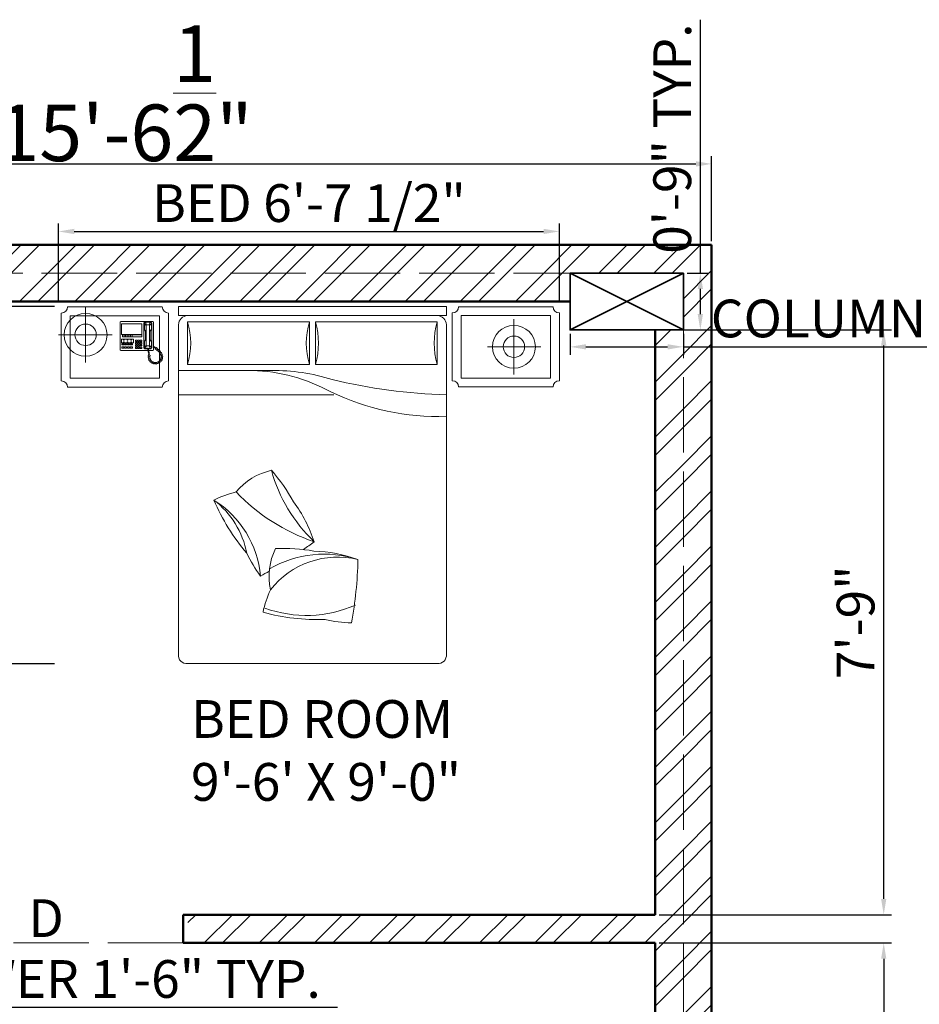
# Model space of a CAD drawing. Units: millimetres. Extents: x 4237 to 5109, y 21391 to 22486.
# Tile 12 of 17: x 4535 to 4678, y 22320 to 22477. Entities that reach past the tile are written whole.
import ezdxf

# ---------------------------------------------------------------- set-up
doc = ezdxf.new("R2010")
doc.units = ezdxf.units.MM
doc.linetypes.add('ACAD_ISO02W100', pattern=[15, 12, -3])
for name, color, linetype, lineweight in [('A-ANNO-DIMS', 2, 'Continuous', 18), ('A-ANNO-TEXT', 7, 'Continuous', 18), ('A-AREA-IDEN', 3, 'Continuous', 18), ('A-FLOR-OVHD', 1, 'ACAD_ISO02W100', 18), ('A-FURN', 8, 'Continuous', 18), ('A-WALL', 7, 'Continuous', 50), ('A-WALL-PATT', 252, 'Continuous', 13), ('column', 102, 'Continuous', 35)]:
    doc.layers.add(name, color=color, linetype=linetype, lineweight=lineweight)
doc.styles.get("Standard").update_dxf_attribs({"font": 'arial.ttf'})
doc.dimstyles.new('ISO-25', dxfattribs={"dimtxt": 6, "dimasz": 2.5, "dimexe": 1.25, "dimexo": 0.625, "dimtad": 1, "dimdec": 1, "dimlunit": 4, "dimtxsty": 'Standard', "dimcen": 2.5, "dimadec": 0, "dimazin": 0, "dimtfac": 1, "dimtdec": 1, "dimtmove": 0, "dimatfit": 3, "dimfxl": 1, "dimarcsym": 0})

# ---------------------------------------------------------------- blocks, each defined once
blk = doc.blocks.new('A$C07097A50')
for p, q in [((0.0503, 1.9981), (0.5803, 1.9981)), ((0.1513, 1.6872), (0.1513, 1.9968)), ((0.6716, 1.9489), (0.6716, 2.0001)), ((0.6716, 2.0001), (2.1719, 2.0001)), ((2.1719, 1.9489), (2.1719, 2.0001)), ((2.7701, 1.9993), (2.2401, 1.9993)), ((0.0153, 1.9631), (0.0153, 1.5831)), ((0.0653, 1.9481), (0.0653, 1.5981)), ((0.0653, 1.9481), (0.5653, 1.9481)), ((0.5653, 1.9481), (0.5653, 1.5981)), ((0.6153, 1.9631), (0.6153, 1.5831)), ((2.1719, 1.9489), (0.6716, 1.9489)), ((2.2051, 1.9643), (2.2051, 1.5843)), ((2.2551, 1.9493), (2.2551, 1.5993)), ((2.7551, 1.9493), (2.2551, 1.9493)), ((2.7551, 1.9493), (2.7551, 1.5993)), ((2.8051, 1.9643), (2.8051, 1.5843)), ((0.3481, 1.9163), (0.3458, 1.914)), ((0.3458, 1.914), (0.3458, 1.7563)), ((0.3481, 1.9163), (0.5287, 1.9163)), ((0.3526, 1.9037), (0.3526, 1.8431)), ((0.4669, 1.9037), (0.3526, 1.9037)), ((0.4669, 1.8431), (0.4669, 1.9037)), ((0.4772, 1.9071), (0.4818, 1.9129)), ((0.4772, 1.7688), (0.4772, 1.9071)), ((0.4818, 1.9094), (0.4807, 1.9049)), ((0.4807, 1.9049), (0.4807, 1.874)), ((0.4807, 1.9049), (0.4909, 1.8946)), ((0.4818, 1.9129), (0.5161, 1.9129)), ((0.4864, 1.9117), (0.4818, 1.9094)), ((0.4921, 1.8969), (0.4864, 1.9117)), ((0.4864, 1.9117), (0.5138, 1.9117)), ((0.4909, 1.8946), (0.4921, 1.8969)), ((0.4909, 1.8431), (0.4909, 1.8946)), ((0.5081, 1.8969), (0.4921, 1.8969)), ((0.5081, 1.8969), (0.5138, 1.9117)), ((0.5092, 1.8946), (0.5081, 1.8969)), ((0.5195, 1.9049), (0.5092, 1.8946)), ((0.5092, 1.8431), (0.5092, 1.8946)), ((0.5138, 1.9117), (0.5184, 1.9094)), ((0.5161, 1.9129), (0.5218, 1.9071)), ((0.5184, 1.9094), (0.5195, 1.9049)), ((0.5195, 1.9049), (0.5195, 1.874)), ((0.5218, 1.9071), (0.5218, 1.77)), ((0.5287, 1.9163), (0.5309, 1.914)), ((0.5309, 1.914), (0.5309, 1.7563)), ((0.6716, 1.8977), (0.6716, 0.0512)), ((2.1719, 0.0512), (2.1719, 1.8977)), ((2.5505, 1.6201), (2.5505, 1.9296)), ((0, 1.8416), (0.3001, 1.8416)), ((0.3526, 1.8431), (0.4669, 1.8431)), ((0.3572, 1.8409), (0.3572, 1.8294)), ((0.4669, 1.8409), (0.3572, 1.8409)), ((0.3572, 1.8294), (0.4669, 1.8294)), ((0.3664, 1.8409), (0.3664, 1.8294)), ((0.3755, 1.8409), (0.3755, 1.8294)), ((0.3846, 1.8409), (0.3846, 1.8294)), ((0.3938, 1.8409), (0.3938, 1.8294)), ((0.4029, 1.8409), (0.4029, 1.8294)), ((0.4121, 1.8409), (0.4121, 1.8294)), ((0.4669, 1.8294), (0.4669, 1.8409)), ((0.4807, 1.874), (0.4829, 1.8683)), ((0.4829, 1.8683), (0.4864, 1.8626)), ((0.4864, 1.8626), (0.4875, 1.8546)), ((0.4864, 1.8134), (0.4875, 1.8214)), ((0.4875, 1.8546), (0.4875, 1.8431)), ((0.4875, 1.8214), (0.4875, 1.8431)), ((0.4909, 1.8431), (0.4909, 1.7814)), ((0.5092, 1.8431), (0.5092, 1.7814)), ((0.5138, 1.8626), (0.5127, 1.8546)), ((0.5127, 1.8546), (0.5127, 1.8431)), ((0.5127, 1.8214), (0.5127, 1.8431)), ((0.5138, 1.8134), (0.5127, 1.8214)), ((0.5172, 1.8683), (0.5138, 1.8626)), ((0.5195, 1.874), (0.5172, 1.8683)), ((0.4201, 1.8168), (0.3526, 1.8168)), ((0.3526, 1.8168), (0.3526, 1.7963)), ((0.3526, 1.7963), (0.4201, 1.7963)), ((0.3652, 1.7906), (0.3538, 1.7906)), ((0.3538, 1.7906), (0.3538, 1.786)), ((0.3538, 1.786), (0.3652, 1.786)), ((0.3538, 1.7666), (0.3538, 1.7734)), ((0.3538, 1.7734), (0.3652, 1.7734)), ((0.3652, 1.7666), (0.3538, 1.7666)), ((0.3675, 1.8146), (0.3641, 1.8146)), ((0.3641, 1.8146), (0.3641, 1.8111)), ((0.3641, 1.8111), (0.3675, 1.8111)), ((0.3641, 1.802), (0.3641, 1.7986)), ((0.3675, 1.802), (0.3641, 1.802)), ((0.3641, 1.7986), (0.3675, 1.7986)), ((0.3652, 1.786), (0.3652, 1.7906)), ((0.3652, 1.7734), (0.3652, 1.7666)), ((0.3675, 1.8111), (0.3675, 1.8146)), ((0.3675, 1.7986), (0.3675, 1.802)), ((0.3812, 1.7906), (0.3698, 1.7906)), ((0.3698, 1.7906), (0.3698, 1.786)), ((0.3698, 1.786), (0.3812, 1.786)), ((0.3698, 1.7666), (0.3698, 1.7734)), ((0.3698, 1.7734), (0.3812, 1.7734)), ((0.3812, 1.7666), (0.3698, 1.7666)), ((0.3812, 1.786), (0.3812, 1.7906)), ((0.3812, 1.7734), (0.3812, 1.7666)), ((0.3846, 1.8146), (0.3846, 1.8111)), ((0.3881, 1.8146), (0.3846, 1.8146)), ((0.3846, 1.8111), (0.3881, 1.8111)), ((0.3846, 1.802), (0.3846, 1.7986)), ((0.3881, 1.802), (0.3846, 1.802)), ((0.3846, 1.7986), (0.3881, 1.7986)), ((0.3972, 1.7906), (0.3858, 1.7906)), ((0.3858, 1.7906), (0.3858, 1.786)), ((0.3858, 1.786), (0.3972, 1.786)), ((0.3858, 1.7666), (0.3858, 1.7734)), ((0.3858, 1.7734), (0.3972, 1.7734)), ((0.3972, 1.7666), (0.3858, 1.7666)), ((0.3881, 1.8111), (0.3881, 1.8146)), ((0.3881, 1.7986), (0.3881, 1.802)), ((0.3972, 1.786), (0.3972, 1.7906)), ((0.3972, 1.7734), (0.3972, 1.7666)), ((0.4018, 1.7906), (0.4018, 1.786)), ((0.4132, 1.7906), (0.4018, 1.7906)), ((0.4018, 1.786), (0.4132, 1.786)), ((0.4018, 1.7734), (0.4132, 1.7734)), ((0.4018, 1.7666), (0.4018, 1.7734)), ((0.4132, 1.7666), (0.4018, 1.7666)), ((0.4052, 1.8146), (0.4052, 1.8111)), ((0.4086, 1.8146), (0.4052, 1.8146)), ((0.4052, 1.8111), (0.4086, 1.8111)), ((0.4052, 1.802), (0.4052, 1.7986)), ((0.4086, 1.802), (0.4052, 1.802)), ((0.4052, 1.7986), (0.4086, 1.7986)), ((0.4086, 1.8111), (0.4086, 1.8146)), ((0.4086, 1.7986), (0.4086, 1.802)), ((0.4132, 1.786), (0.4132, 1.7906)), ((0.4132, 1.7734), (0.4132, 1.7666)), ((0.4201, 1.7963), (0.4201, 1.8168)), ((0.4304, 1.8111), (0.4395, 1.8111)), ((0.4304, 1.8043), (0.4304, 1.8111)), ((0.4395, 1.8043), (0.4304, 1.8043)), ((0.4304, 1.7986), (0.4395, 1.7986)), ((0.4304, 1.7917), (0.4304, 1.7986)), ((0.4395, 1.7917), (0.4304, 1.7917)), ((0.4304, 1.778), (0.4304, 1.7848)), ((0.4304, 1.7848), (0.4395, 1.7848)), ((0.4395, 1.778), (0.4304, 1.778)), ((0.4304, 1.7723), (0.4395, 1.7723)), ((0.4304, 1.7654), (0.4304, 1.7723)), ((0.4395, 1.8111), (0.4395, 1.8043)), ((0.4395, 1.7986), (0.4395, 1.7917)), ((0.4395, 1.7848), (0.4395, 1.778)), ((0.4395, 1.7723), (0.4395, 1.7654)), ((0.4441, 1.8043), (0.4441, 1.8111)), ((0.4441, 1.8111), (0.4532, 1.8111)), ((0.4532, 1.8043), (0.4441, 1.8043)), ((0.4441, 1.7986), (0.4532, 1.7986)), ((0.4441, 1.7917), (0.4441, 1.7986)), ((0.4532, 1.7917), (0.4441, 1.7917)), ((0.4441, 1.778), (0.4441, 1.7848)), ((0.4441, 1.7848), (0.4532, 1.7848)), ((0.4532, 1.778), (0.4441, 1.778)), ((0.4441, 1.7723), (0.4532, 1.7723)), ((0.4441, 1.7654), (0.4441, 1.7723)), ((0.4532, 1.8111), (0.4532, 1.8043)), ((0.4532, 1.7986), (0.4532, 1.7917)), ((0.4532, 1.7848), (0.4532, 1.778)), ((0.4532, 1.7723), (0.4532, 1.7654)), ((0.4578, 1.8111), (0.4669, 1.8111)), ((0.4578, 1.8043), (0.4578, 1.8111)), ((0.4669, 1.8043), (0.4578, 1.8043)), ((0.4578, 1.7986), (0.4669, 1.7986)), ((0.4578, 1.7917), (0.4578, 1.7986)), ((0.4669, 1.7917), (0.4578, 1.7917)), ((0.4578, 1.7791), (0.4578, 1.786)), ((0.4578, 1.786), (0.4669, 1.786)), ((0.4669, 1.7791), (0.4578, 1.7791)), ((0.4578, 1.7654), (0.4578, 1.7723)), ((0.4578, 1.7723), (0.4669, 1.7723)), ((0.4669, 1.8111), (0.4669, 1.8043)), ((0.4669, 1.7986), (0.4669, 1.7917)), ((0.4669, 1.786), (0.4669, 1.7791)), ((0.4669, 1.7723), (0.4669, 1.7654)), ((0.4829, 1.7631), (0.4772, 1.7688)), ((0.4807, 1.802), (0.4829, 1.8077)), ((0.4807, 1.7711), (0.4807, 1.802)), ((0.4807, 1.7711), (0.4909, 1.7814)), ((0.4818, 1.7666), (0.4807, 1.7711)), ((0.4864, 1.7643), (0.4818, 1.7666)), ((0.4829, 1.8077), (0.4864, 1.8134)), ((0.4921, 1.7791), (0.4864, 1.7643)), ((0.4909, 1.7814), (0.4921, 1.7791)), ((0.5081, 1.7791), (0.4921, 1.7791)), ((0.5024, 1.7677), (0.4989, 1.7677)), ((0.4989, 1.7677), (0.4991, 1.7578)), ((0.503, 1.7585), (0.5024, 1.7677)), ((0.5092, 1.7814), (0.5081, 1.7791)), ((0.5081, 1.7791), (0.5138, 1.7643)), ((0.5195, 1.7711), (0.5092, 1.7814)), ((0.5172, 1.8077), (0.5138, 1.8134)), ((0.5138, 1.7643), (0.5184, 1.7666)), ((0.5218, 1.77), (0.5161, 1.7631)), ((0.5195, 1.802), (0.5172, 1.8077)), ((0.5184, 1.7666), (0.5195, 1.7711)), ((0.5195, 1.7711), (0.5195, 1.802)), ((0.5378, 1.7743), (0.5309, 1.7768)), ((0.5309, 1.7723), (0.536, 1.7709)), ((0.536, 1.7709), (0.5406, 1.7672)), ((0.541, 1.7711), (0.5378, 1.7743)), ((0.5406, 1.7672), (0.5418, 1.7656)), ((0.5434, 1.7689), (0.541, 1.7711)), ((0.5442, 1.7658), (0.5418, 1.7634)), ((0.5418, 1.7656), (0.5442, 1.7658)), ((0.5477, 1.7705), (0.5434, 1.7689)), ((0.5497, 1.7685), (0.5477, 1.7705)), ((0.5481, 1.765), (0.5497, 1.7685)), ((0.5509, 1.7672), (0.5481, 1.765)), ((0.5539, 1.764), (0.5509, 1.7672)), ((2.7018, 1.7745), (2.4017, 1.7745)), ((0.3458, 1.7563), (0.3481, 1.754)), ((0.5, 1.754), (0.3481, 1.754)), ((0.4395, 1.7654), (0.4304, 1.7654)), ((0.4532, 1.7654), (0.4441, 1.7654)), ((0.4669, 1.7654), (0.4578, 1.7654)), ((0.499, 1.7631), (0.4829, 1.7631)), ((0.4864, 1.7643), (0.499, 1.7643)), ((0.4991, 1.7578), (0.5019, 1.7463)), ((0.5019, 1.7463), (0.5047, 1.7354)), ((0.5026, 1.7254), (0.5021, 1.7199)), ((0.5021, 1.7199), (0.5088, 1.7187)), ((0.5088, 1.7187), (0.5023, 1.7148)), ((0.5023, 1.7148), (0.5028, 1.7085)), ((0.5026, 1.7643), (0.5138, 1.7643)), ((0.5051, 1.728), (0.5026, 1.7254)), ((0.5161, 1.7631), (0.5027, 1.7631)), ((0.5047, 1.7511), (0.503, 1.7585)), ((0.5287, 1.754), (0.504, 1.754)), ((0.5047, 1.7354), (0.5044, 1.7294)), ((0.5044, 1.7294), (0.5051, 1.728)), ((0.5074, 1.7403), (0.5047, 1.7511)), ((0.5081, 1.7347), (0.5074, 1.7403)), ((0.5079, 1.7287), (0.5081, 1.7347)), ((0.5121, 1.7257), (0.5079, 1.7287)), ((0.5111, 1.7203), (0.5121, 1.7257)), ((0.5123, 1.7058), (0.5111, 1.7203)), ((0.5309, 1.7563), (0.5287, 1.754)), ((0.5418, 1.7634), (0.5511, 1.7552)), ((0.5511, 1.7552), (0.5662, 1.7423)), ((0.5515, 1.7574), (0.5539, 1.764)), ((0.5577, 1.7606), (0.5515, 1.7574)), ((0.563, 1.7556), (0.5577, 1.7606)), ((0.5618, 1.7483), (0.563, 1.7556)), ((0.567, 1.7515), (0.5618, 1.7483)), ((0.5664, 1.7419), (0.574, 1.7201)), ((0.5714, 1.7469), (0.567, 1.7515)), ((0.5696, 1.7419), (0.5714, 1.7469)), ((0.5766, 1.7426), (0.5697, 1.7419)), ((0.574, 1.7201), (0.5708, 1.7028)), ((0.572, 1.7331), (0.5787, 1.7356)), ((0.5794, 1.7333), (0.572, 1.7331)), ((0.5761, 1.7234), (0.581, 1.728)), ((0.5824, 1.7234), (0.5761, 1.7234)), ((0.5764, 1.7155), (0.5835, 1.7176)), ((0.5824, 1.712), (0.5764, 1.7155)), ((0.5787, 1.7356), (0.5766, 1.7426)), ((0.581, 1.728), (0.5794, 1.7333)), ((0.5814, 1.7074), (0.5824, 1.712)), ((0.5835, 1.7176), (0.5824, 1.7234)), ((0.5028, 1.7085), (0.5102, 1.7078)), ((0.5102, 1.7078), (0.5037, 1.7028)), ((0.5037, 1.7028), (0.5067, 1.6974)), ((0.5067, 1.6974), (0.5137, 1.6988)), ((0.5137, 1.6988), (0.5104, 1.6923)), ((0.5104, 1.6923), (0.5139, 1.6882)), ((0.5211, 1.6947), (0.5123, 1.7058)), ((0.5139, 1.6882), (0.5192, 1.6921)), ((0.5192, 1.6921), (0.5183, 1.6859)), ((0.5183, 1.6859), (0.5227, 1.6831)), ((0.5333, 1.6882), (0.5211, 1.6947)), ((0.5227, 1.6831), (0.5282, 1.6877)), ((0.5282, 1.6877), (0.5276, 1.6801)), ((0.5276, 1.6801), (0.5324, 1.6787)), ((0.5324, 1.6787), (0.5354, 1.6849)), ((0.5472, 1.687), (0.5333, 1.6882)), ((0.5354, 1.6849), (0.5382, 1.6787)), ((0.5382, 1.6787), (0.5421, 1.6782)), ((0.5421, 1.6782), (0.5437, 1.6849)), ((0.5437, 1.6849), (0.5463, 1.6775)), ((0.5463, 1.6775), (0.5507, 1.6787)), ((0.5606, 1.6928), (0.5472, 1.687)), ((0.5507, 1.6787), (0.5509, 1.6849)), ((0.5509, 1.6849), (0.5562, 1.6803)), ((0.5562, 1.6803), (0.5599, 1.6822)), ((0.5592, 1.6891), (0.5641, 1.6831)), ((0.5599, 1.6822), (0.5592, 1.6891)), ((0.5708, 1.7028), (0.5606, 1.6928)), ((0.5641, 1.6831), (0.5678, 1.6863)), ((0.565, 1.6926), (0.5715, 1.6898)), ((0.5678, 1.6863), (0.565, 1.6926)), ((0.5745, 1.6926), (0.5713, 1.6988)), ((0.5713, 1.6988), (0.578, 1.6967)), ((0.5715, 1.6898), (0.5745, 1.6926)), ((0.5743, 1.7076), (0.5814, 1.7074)), ((0.5798, 1.7014), (0.5743, 1.7076)), ((0.578, 1.6967), (0.5798, 1.7014)), ((0.0503, 1.5481), (0.5803, 1.5481)), ((0.0653, 1.5981), (0.5653, 1.5981)), ((2.7701, 1.5493), (2.2401, 1.5493)), ((2.7551, 1.5993), (2.2551, 1.5993)), ((0.7228, 0.0001), (2.1207, 0.0001))]:
    blk.add_line(p, q)
at = {"linetype": 'ByBlock'}
for p, q in [((0.7228, 1.6759), (0.7228, 1.9148)), ((0.7228, 1.9148), (1.4047, 1.9148)), ((1.4047, 1.9148), (1.4047, 1.6759)), ((1.4388, 1.6759), (1.4388, 1.9148)), ((1.4388, 1.9148), (2.1207, 1.9148)), ((2.1207, 1.9148), (2.1207, 1.6759)), ((1.4047, 1.6759), (0.7228, 1.6759)), ((2.1207, 1.6759), (1.4388, 1.6759)), ((1.1914, 1.6418), (0.6716, 1.6418)), ((1.5412, 1.5053), (0.6716, 1.5053))]:
    blk.add_line(p, q, dxfattribs=at)
for centre in [(0.1513, 1.8416), (2.5505, 1.7745)]:
    blk.add_circle(centre, 0.12, dxfattribs=at)
for centre in [(0.1513, 1.8416), (2.5505, 1.7745)]:
    blk.add_circle(centre, 0.06)
for centre, radius, start, end in [((0.0153, 1.9981), 0.035, 270, 0), ((0.6153, 1.9981), 0.035, 180, 270), ((2.2051, 1.9993), 0.035, 270, 0), ((2.8051, 1.9993), 0.035, 180, 270), ((0.7228, 1.8977), 0.0512, 90, 180), ((2.1207, 1.8977), 0.0512, 0, 90), ((0.0153, 1.5481), 0.035, 0, 90), ((0.6153, 1.5481), 0.035, 90, 180), ((2.2051, 1.5493), 0.035, 0, 90), ((2.8051, 1.5493), 0.035, 90, 180), ((1.2698, 0.7333), 0.3575, 102.4782, 140.4625), ((0.4476, 0.4335), 0.9879, 28.4971, 41.0566), ((2.0313, 1.3124), 0.8697, 195.336, 226.4193), ((1.1192, 0.4274), 0.548, 103.2034, 117.0362), ((1.7756, 1.7059), 1.0798, 223.6306, 251.4288), ((1.9422, 1.372), 1.1652, 203.0642, 220.3209), ((0.5744, 0.5274), 0.4879, 10.6986, 52.6864), ((0.5678, 0.4375), 0.5655, 5.3391, 57.6895), ((0.6844, 0.4345), 0.7874, 18.3527, 36.6851), ((0.1017, 2.4319), 2.1977, 305.2966, 307.2418), ((1.7177, 0.9312), 0.734, 205.259, 216.9351), ((1.5362, 0.487), 0.3575, 154.0418, 192.0262), ((1.4868, 0.0041), 0.6085, 71.81, 120.1351), ((1.2599, -0.3434), 0.9879, 80.0607, 92.6202), ((1.4063, -0.1573), 0.7874, 69.9163, 88.2487), ((1.5627, 0.1186), 0.4774, 76.1849, 142.0017), ((-0.5205, 0.628), 2.1977, 349.4884, 358.8054), ((0.1017, 2.4319), 2.1977, 297.9248, 299.3793), ((1.6822, 0.1789), 0.548, 154.767, 168.5998), ((1.4539, 1.4107), 1.1652, 254.6278, 271.8845), ((1.3874, 0.9578), 0.6885, 250.2936, 293.6414), ((1.6595, 0.9609), 0.734, 256.8226, 268.4988), ((0.717, 0.0455), 0.0458, 172.7599, 277.2401), ((2.1265, 0.0455), 0.0458, 262.7599, 7.2401)]:
    blk.add_arc(centre, radius, start, end)
for centre, radius, start, end in [((0.3133, 1.7953), 0.4265, 343.7398, 16.2602), ((1.8141, 1.7953), 0.4265, 163.7398, 196.2602), ((1.0294, 1.7953), 0.4265, 343.7398, 16.2602), ((2.5302, 1.7953), 0.4265, 163.7398, 196.2602), ((1.053, 0.6571), 0.9853, 61.4328, 88.1261), ((1.2053, 0.5713), 1.0706, 72.1966, 90.7418), ((2.2595, 4.5996), 3.0955, 256.4201, 268.3789), ((2.1283, 2.7745), 1.3903, 244.2427, 271.7984)]:
    blk.add_arc(centre, radius, start, end, dxfattribs=at)
blk = doc.blocks.new('*D57')
at = {"layer": 'A-ANNO-DIMS', "color": 0, "lineweight": -2, "transparency": 16777216}
for p, q in [((4458.3, 22441.33), (4458.3, 22454.84)), ((4644.95, 22441.33), (4644.95, 22454.84)), ((4460.8, 22453.59), (4642.45, 22453.59))]:
    blk.add_line(p, q, dxfattribs=at)
at = {"layer": 'A-ANNO-DIMS', "color": 0, "transparency": 16777216}
for points in [[(4460.8, 22454.01), (4460.8, 22453.17), (4458.3, 22453.59)], [(4642.45, 22454.01), (4642.45, 22453.17), (4644.95, 22453.59)]]:
    blk.add_solid(points, dxfattribs=at)
at = {"layer": 'Defpoints', "color": 0, "transparency": 16777216}
for p in [(4644.95, 22453.59), (4458.3, 22440.7), (4644.95, 22440.7)]:
    blk.add_point(p, dxfattribs=at)
at = {"layer": 'A-ANNO-DIMS', "color": 0, "transparency": 16777216, "insert": (4551.63, 22464.83), "char_height": 9, "attachment_point": 5}
blk.add_mtext('15\'-6{\\H1x;\\S1/2;}"', dxfattribs=at)
blk = doc.blocks.new('COLUMN-X')
blk.add_line((18, 9), (0, 0))
blk.add_lwpolyline([(18, 9), (0, 9), (0, 0), (18, 0)], close=True)
blk = doc.blocks.new('*D66')
at = {"layer": 'A-ANNO-DIMS', "color": 0, "lineweight": -2, "transparency": 16777216}
for p, q in [((4541.13, 22431.53), (4541.13, 22444.1)), ((4620.74, 22431.53), (4620.74, 22444.1)), ((4543.63, 22442.85), (4618.24, 22442.85))]:
    blk.add_line(p, q, dxfattribs=at)
at = {"layer": 'A-ANNO-DIMS', "color": 0, "transparency": 16777216}
for points in [[(4543.63, 22443.27), (4543.63, 22442.43), (4541.13, 22442.85)], [(4618.24, 22443.27), (4618.24, 22442.43), (4620.74, 22442.85)]]:
    blk.add_solid(points, dxfattribs=at)
at = {"layer": 'Defpoints', "color": 0, "transparency": 16777216}
for p in [(4620.74, 22442.85), (4541.13, 22430.91), (4620.74, 22430.91)]:
    blk.add_point(p, dxfattribs=at)
at = {"layer": 'A-ANNO-DIMS', "color": 0, "transparency": 16777216, "insert": (4580.94, 22446.58), "char_height": 6, "attachment_point": 5}
blk.add_mtext('BED 6\'-7 1/2"', dxfattribs=at)
blk = doc.blocks.new('*D67')
at = {"layer": 'A-ANNO-DIMS', "color": 0, "lineweight": -2, "transparency": 16777216}
for p, q in [((4540.51, 22430.91), (4527.94, 22430.91)), ((4529.19, 22376.6), (4529.19, 22428.41)), ((4540.51, 22374.1), (4527.94, 22374.1))]:
    blk.add_line(p, q, dxfattribs=at)
at = {"layer": 'A-ANNO-DIMS', "color": 0, "transparency": 16777216}
for points in [[(4528.78, 22428.41), (4529.61, 22428.41), (4529.19, 22430.91)], [(4528.78, 22376.6), (4529.61, 22376.6), (4529.19, 22374.1)]]:
    blk.add_solid(points, dxfattribs=at)
at = {"layer": 'Defpoints', "color": 0, "transparency": 16777216}
for p in [(4529.19, 22430.91), (4541.13, 22430.91), (4541.13, 22374.1)]:
    blk.add_point(p, dxfattribs=at)
at = {"layer": 'A-ANNO-DIMS', "color": 0, "transparency": 16777216, "insert": (4525.5, 22402.5), "char_height": 6, "attachment_point": 5, "rotation": 90}
blk.add_mtext('4\'-9"', dxfattribs=at)
blk = doc.blocks.new('*D78')
at = {"layer": 'A-ANNO-DIMS', "color": 0, "lineweight": -2, "transparency": 16777216}
for p, q in [((4622.45, 22426.58), (4622.45, 22423.25)), ((4640.45, 22426.58), (4640.45, 22423.25)), ((4624.95, 22424.5), (4637.95, 22424.5)), ((4640.45, 22424.5), (4719.36, 22424.5))]:
    blk.add_line(p, q, dxfattribs=at)
at = {"layer": 'A-ANNO-DIMS', "color": 0, "transparency": 16777216}
for points in [[(4624.95, 22424.92), (4624.95, 22424.08), (4622.45, 22424.5)], [(4637.95, 22424.92), (4637.95, 22424.08), (4640.45, 22424.5)]]:
    blk.add_solid(points, dxfattribs=at)
at = {"layer": 'Defpoints', "color": 0, "transparency": 16777216}
for p in [(4622.45, 22427.2), (4640.45, 22427.2), (4640.45, 22424.5)]:
    blk.add_point(p, dxfattribs=at)
at = {"layer": 'A-ANNO-DIMS', "color": 0, "transparency": 16777216, "insert": (4681.15, 22428.23), "char_height": 6, "attachment_point": 5}
blk.add_mtext('COLUMN 1\'-6" TYP.', dxfattribs=at)
blk = doc.blocks.new('*D79')
at = {"layer": 'A-ANNO-DIMS', "color": 0, "lineweight": -2, "transparency": 16777216}
for p, q in [((4643.15, 22436.2), (4643.15, 22476.52)), ((4641.08, 22436.2), (4644.4, 22436.2)), ((4643.15, 22429.7), (4643.15, 22433.7)), ((4641.08, 22427.2), (4644.4, 22427.2))]:
    blk.add_line(p, q, dxfattribs=at)
at = {"layer": 'A-ANNO-DIMS', "color": 0, "transparency": 16777216}
for points in [[(4642.73, 22433.7), (4643.57, 22433.7), (4643.15, 22436.2)], [(4642.73, 22429.7), (4643.57, 22429.7), (4643.15, 22427.2)]]:
    blk.add_solid(points, dxfattribs=at)
at = {"layer": 'Defpoints', "color": 0, "transparency": 16777216}
for p in [(4640.45, 22436.2), (4643.15, 22436.2), (4640.45, 22427.2)]:
    blk.add_point(p, dxfattribs=at)
at = {"layer": 'A-ANNO-DIMS', "color": 0, "transparency": 16777216, "insert": (4639.46, 22457.61), "char_height": 6, "attachment_point": 5, "rotation": 90}
blk.add_mtext('0\'-9" TYP.', dxfattribs=at)
blk = doc.blocks.new('*D90')
at = {"layer": 'A-ANNO-DIMS', "color": 0, "lineweight": -2, "transparency": 16777216}
for p, q in [((4486.92, 22321.58), (4486.92, 22318.22)), ((4505.11, 22321.58), (4505.11, 22318.22)), ((4489.42, 22319.47), (4502.61, 22319.47)), ((4505.11, 22319.47), (4585.45, 22319.47))]:
    blk.add_line(p, q, dxfattribs=at)
at = {"layer": 'A-ANNO-DIMS', "color": 0, "transparency": 16777216}
for points in [[(4489.42, 22319.89), (4489.42, 22319.06), (4486.92, 22319.47)], [(4502.61, 22319.89), (4502.61, 22319.06), (4505.11, 22319.47)]]:
    blk.add_solid(points, dxfattribs=at)
at = {"layer": 'Defpoints', "color": 0, "transparency": 16777216}
for p in [(4486.92, 22322.2), (4505.11, 22322.2), (4505.11, 22319.47)]:
    blk.add_point(p, dxfattribs=at)
at = {"layer": 'A-ANNO-DIMS', "color": 0, "transparency": 16777216, "insert": (4546.53, 22323.2), "char_height": 6, "attachment_point": 5}
blk.add_mtext('SHOWER 1\'-6" TYP.', dxfattribs=at)
blk = doc.blocks.new('*D105')
at = {"layer": 'A-ANNO-DIMS', "color": 0, "lineweight": -2, "transparency": 16777216}
for p, q in [((4636.58, 22427.2), (4673.55, 22427.2)), ((4672.3, 22336.7), (4672.3, 22424.7)), ((4636.58, 22334.2), (4673.55, 22334.2))]:
    blk.add_line(p, q, dxfattribs=at)
at = {"layer": 'A-ANNO-DIMS', "color": 0, "transparency": 16777216}
for points in [[(4671.88, 22424.7), (4672.72, 22424.7), (4672.3, 22427.2)], [(4671.88, 22336.7), (4672.72, 22336.7), (4672.3, 22334.2)]]:
    blk.add_solid(points, dxfattribs=at)
at = {"layer": 'Defpoints', "color": 0, "transparency": 16777216}
for p in [(4635.95, 22427.2), (4672.3, 22427.2), (4635.95, 22334.2)]:
    blk.add_point(p, dxfattribs=at)
at = {"layer": 'A-ANNO-DIMS', "color": 0, "transparency": 16777216, "insert": (4668.61, 22380.7), "char_height": 6, "attachment_point": 5, "rotation": 90}
blk.add_mtext('7\'-9"', dxfattribs=at)
blk = doc.blocks.new('*D106')
at = {"layer": 'A-ANNO-DIMS', "color": 0, "lineweight": -2, "transparency": 16777216}
for p, q in [((4636.58, 22329.7), (4673.55, 22329.7)), ((4672.3, 22327.2), (4672.3, 22240.7)), ((4636.58, 22238.2), (4673.55, 22238.2))]:
    blk.add_line(p, q, dxfattribs=at)
at = {"layer": 'A-ANNO-DIMS', "color": 0, "transparency": 16777216}
for points in [[(4671.88, 22327.2), (4672.72, 22327.2), (4672.3, 22329.7)], [(4671.88, 22240.7), (4672.72, 22240.7), (4672.3, 22238.2)]]:
    blk.add_solid(points, dxfattribs=at)
at = {"layer": 'Defpoints', "color": 0, "transparency": 16777216}
for p in [(4635.95, 22329.7), (4635.95, 22238.2), (4672.3, 22238.2)]:
    blk.add_point(p, dxfattribs=at)
at = {"layer": 'A-ANNO-DIMS', "color": 0, "transparency": 16777216, "insert": (4668.57, 22283.95), "char_height": 6, "attachment_point": 5, "rotation": 90}
blk.add_mtext('7\'-7 1/2"', dxfattribs=at)

msp = doc.modelspace()

# ---------------------------------------------------------------- hatches: boundary and pattern name
at = {"layer": 'A-WALL-PATT'}
h = msp.add_hatch(dxfattribs=at)
h.set_pattern_fill('ANSI32', color=256, scale=0.65)
h.paths.add_polyline_path([(4644.95, 22440.7), (4517.45, 22440.7), (4517.45, 22436.2), (4622.45, 22436.2), (4640.45, 22436.2), (4640.45, 22427.2), (4640.45, 22233.7), (4644.95, 22233.7)])
h = msp.add_hatch(dxfattribs=at)
h.set_pattern_fill('ANSI32', color=256, scale=0.65)
h.paths.add_polyline_path([(4622.45, 22436.2), (4517.45, 22436.2), (4517.45, 22431.7), (4521.95, 22431.7), (4622.45, 22431.7)], flags=17)
h = msp.add_hatch(dxfattribs=at)
h.set_pattern_fill('ANSI32', color=256, scale=0.65)
h.paths.add_polyline_path([(4640.45, 22427.2), (4635.95, 22427.2), (4635.95, 22334.2), (4560.95, 22334.2), (4560.95, 22332.95), (4561.95, 22332.95), (4561.95, 22332.56), (4562.47, 22332.56), (4562.47, 22331.34), (4561.95, 22331.34), (4561.95, 22330.95), (4560.95, 22330.95), (4560.95, 22329.7), (4635.95, 22329.7), (4635.95, 22311.7), (4640.45, 22311.7)], flags=17)

# ---------------------------------------------------------------- linework, layer by layer
at = {"layer": 'A-FLOR-OVHD'}
msp.add_line((4560.95, 22329.7), (4521.95, 22329.7), dxfattribs=at)
msp.add_lwpolyline([(4640.45, 22032.7), (4640.45, 22436.2), (4276.15, 22436.2), (4276.15, 22032.7)], dxfattribs=at)
at = {"layer": 'A-WALL'}
for p, q in [((4271.65, 22440.7), (4644.95, 22440.7)), ((4644.95, 22440.7), (4644.95, 22032.7)), ((4521.95, 22431.7), (4622.45, 22431.7)), ((4635.95, 22427.2), (4635.95, 22334.2)), ((4560.95, 22334.2), (4635.95, 22334.2)), ((4560.95, 22334.2), (4560.95, 22329.7)), ((4560.95, 22329.7), (4635.95, 22329.7)), ((4635.95, 22329.7), (4635.95, 22311.7))]:
    msp.add_line(p, q, dxfattribs=at)
at = {"layer": 'column'}
msp.add_line((4622.45, 22436.2), (4640.45, 22427.2), dxfattribs=at)

# ---------------------------------------------------------------- block references
at = {"layer": 'A-FURN', "xscale": 28.37925203824453, "yscale": 28.37925203824453, "zscale": 28.37925203824453}
msp.add_blockref('A$C07097A50', (4541.14, 22374.15), dxfattribs=at)
at = {"layer": 'column'}
msp.add_blockref('COLUMN-X', (4622.45, 22427.2), dxfattribs=at)

# ---------------------------------------------------------------- texts
at = {"layer": 'A-ANNO-TEXT', "insert": (4529, 22336.65), "char_height": 6, "attachment_point": 1}
msp.add_mtext_dynamic_manual_height_columns('    D', width=21.7253, gutter_width=12.5, heights=[0], dxfattribs=at)
at = {"layer": 'A-AREA-IDEN', "insert": (4562.19, 22368.32), "char_height": 6, "attachment_point": 1}
msp.add_mtext_dynamic_manual_height_columns('BED ROOM \\P9\'-6\' X 9\'-0"', width=55.7646, gutter_width=12.5, heights=[0], dxfattribs=at)

# ---------------------------------------------------------------- dimensions: what is measured, and where the dimension line sits
at = {"layer": 'A-ANNO-DIMS'}
dim = msp.add_linear_dim(base=(4643.15, 22436.2), p1=(4640.45, 22427.2), p2=(4640.45, 22436.2), angle=90, text='<> TYP.', dimstyle='ISO-25', override={"dimdec": 1, "dimrnd": 0, "dimzin": 1, "dimlunit": 4, "dimfrac": 2}, dxfattribs=at)
dim.commit()
dim.dimension.update_dxf_attribs({"geometry": '*D79', "text_midpoint": (4639.46, 22457.61)})
dim = msp.add_linear_dim(base=(4644.95138825, 22453.59015802), p1=(4458.30138825, 22440.70062861), p2=(4644.95138825, 22440.70062861), dimstyle='ISO-25', override={"dimtxt": 9, "dimclrd": 0, "dimclre": 0, "dimclrt": 0}, dxfattribs=at)
dim.commit()
dim.dimension.update_dxf_attribs({"geometry": '*D57', "text_midpoint": (4551.62638825, 22464.82873237)})
for base, p1, p2, text, picture, middle in [((4620.74, 22442.85), (4541.13, 22430.91), (4620.74, 22430.91), 'BED <>', '*D66', (4580.94, 22446.58)), ((4640.45, 22424.5), (4622.45, 22427.2), (4640.45, 22427.2), 'COLUMN <> TYP.', '*D78', (4681.15, 22428.23)), ((4505.11, 22319.47), (4486.92, 22322.2), (4505.11, 22322.2), 'SHOWER <> TYP.', '*D90', (4546.53, 22323.2))]:
    dim = msp.add_linear_dim(base=base, p1=p1, p2=p2, text=text, dimstyle='ISO-25', override={"dimdec": 1, "dimrnd": 0, "dimzin": 1, "dimlunit": 4, "dimfrac": 2}, dxfattribs=at)
    dim.commit()
    dim.dimension.update_dxf_attribs({"geometry": picture, "text_midpoint": middle})
for base, p1, p2, override, picture, middle in [((4529.19, 22430.91), (4541.13, 22374.1), (4541.13, 22430.91), {"dimdec": 1, "dimrnd": 0, "dimzin": 1, "dimlunit": 4, "dimfrac": 2}, '*D67', (4525.5, 22402.5)), ((4672.3, 22427.2), (4635.95, 22334.2), (4635.95, 22427.2), {"dimdec": 1, "dimlfac": 1, "dimrnd": 0, "dimzin": 1, "dimdsep": 46, "dimlunit": 4, "dimfrac": 2}, '*D105', (4668.61, 22380.7)), ((4672.3, 22238.2), (4635.95, 22329.7), (4635.95, 22238.2), {"dimdec": 1, "dimlfac": 1, "dimrnd": 0, "dimzin": 1, "dimdsep": 46, "dimlunit": 4, "dimfrac": 2}, '*D106', (4668.57, 22283.95))]:
    dim = msp.add_linear_dim(base=base, p1=p1, p2=p2, angle=90, dimstyle='ISO-25', override=override, dxfattribs=at)
    dim.commit()
    dim.dimension.update_dxf_attribs({"geometry": picture, "text_midpoint": middle})

doc.saveas('drawing.dxf')
